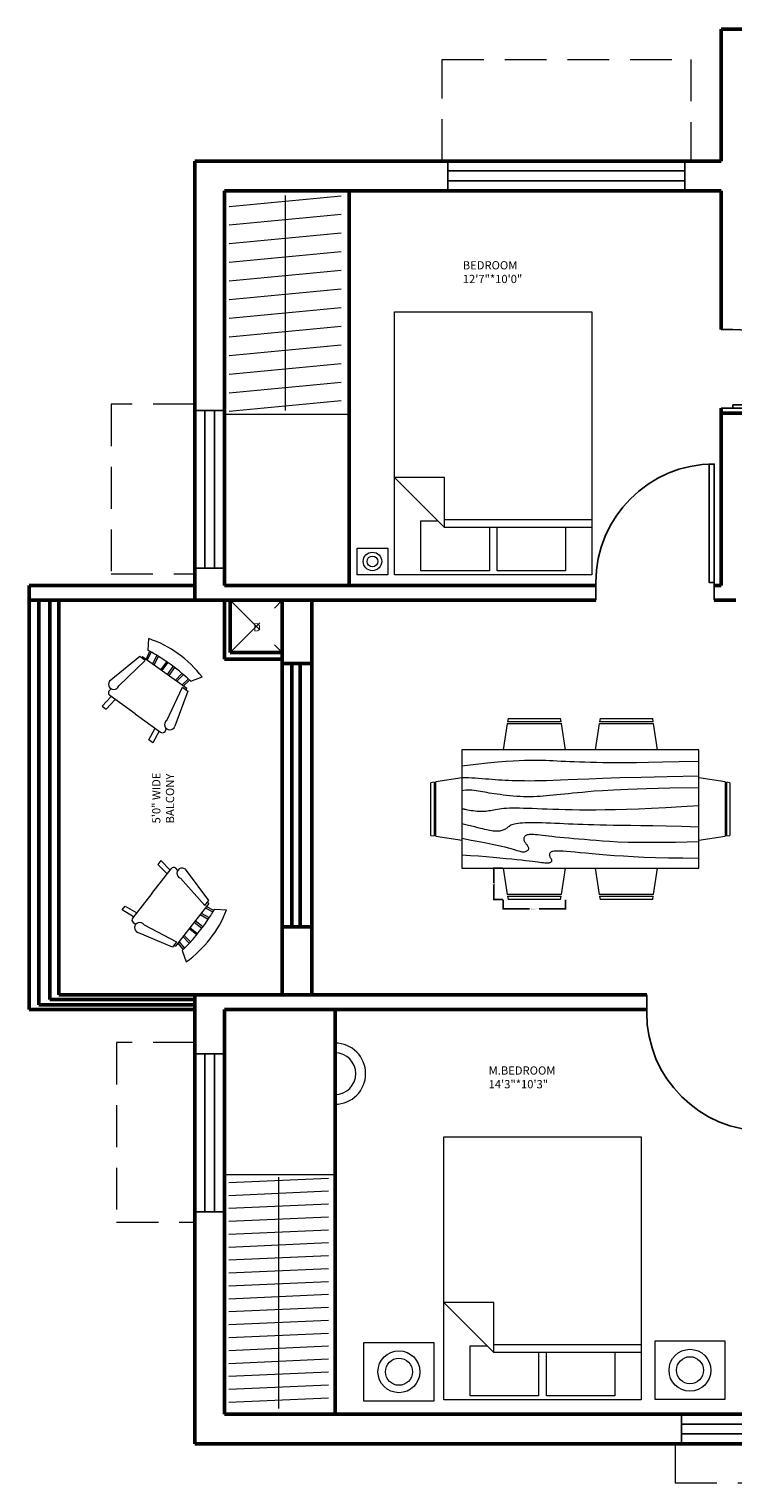
# Model space of a CAD drawing. Units: inches. Extents: x 4795 to 6024, y 2716 to 5025.
# Tile 4 of 19: x 4867 to 5081, y 3339 to 3781. Entities that reach past the tile are written whole.
import ezdxf

# ---------------------------------------------------------------- set-up
doc = ezdxf.new("R2010")
doc.units = ezdxf.units.IN
doc.linetypes.add('DASHED', pattern=[19.05, 12.7, -6.35])
for name, color, linetype, lineweight in [('A-ANNO-DIMS', 2, 'Continuous', 18), ('A-ANNO-TEXT', 7, 'Continuous', 18), ('A-AREA-IDEN', 3, 'Continuous', 18), ('A-DOOR', 4, 'Continuous', 25), ('A-FLOR-FIXT', 9, 'Continuous', 18), ('A-FURN', 8, 'Continuous', 18), ('A-GLAZ', 4, 'Continuous', 25), ('A-WALL', 7, 'Continuous', 50), ('A-WALL-OVHD', 8, 'DASHED', 18)]:
    doc.layers.add(name, color=color, linetype=linetype, lineweight=lineweight)
doc.styles.get("Standard").update_dxf_attribs({"font": 'arial.ttf'})
doc.dimstyles.get("Standard").update_dxf_attribs({"dimtxt": 0.18, "dimasz": 0.18, "dimexe": 0.18, "dimexo": 0.0625, "dimgap": 0.09, "dimtad": 0, "dimtih": 1, "dimtoh": 1, "dimdec": 4, "dimzin": 0, "dimdsep": 46, "dimtxsty": 'Standard', "dimcen": 0.09, "dimadec": 0, "dimazin": 0, "dimtfac": 1, "dimtdec": 4, "dimtofl": 0, "dimtmove": 0, "dimatfit": 3, "dimfxl": 1, "dimtolj": 1, "dimtzin": 0, "dimarcsym": 0})

# ---------------------------------------------------------------- blocks, each defined once
blk = doc.blocks.new('*U2')
for p, q in [((0, 0), (0, -6)), ((40, 0), (40, -6))]:
    blk.add_line(p, q)
blk.add_lwpolyline([(0, 0), (0, 40), (1.75, 40), (1.75, 0)], close=True)
blk.add_arc((0, 0), 40, 0, 90)
blk = doc.blocks.new('Bed - Queen')
for p, q in [((0, -80.00003), (0, 0)), ((0, 0), (59.99999, 0)), ((59.99999, 0), (59.99999, -80.00003)), ((7.99999, -1.2), (28.79998, -1.2)), ((7.99999, -14.4), (7.99999, -1.2)), ((28.79998, -1.2), (28.79998, -14.4)), ((31.19999, -1.2), (51.99999, -1.2)), ((31.19999, -14.4), (31.19999, -1.2)), ((51.99999, -1.2), (51.99999, -16.4)), ((0, -14.4), (44.8, -14.4)), ((44.8, -16.8), (0, -16.8)), ((59.99999, -29.6), (44.8, -14.4)), ((44.8, -14.4), (44.8, -29.6)), ((51.99999, -16.4), (46.79936, -16.4)), ((44.8, -29.6), (59.99999, -29.6)), ((59.99999, -80.00003), (0, -80.00003))]:
    blk.add_line(p, q)
blk = doc.blocks.new('Chair - Rocking')
for p, q in [((-8, -4.5), (-10, -1.5)), ((-4.5, -7), (-4.96674, -4.19951)), ((-4, -7), (-4.40532, -4.16272)), ((-1.5, -4.05012), (-1.5, -7)), ((-1, -7), (-1, -4.05012)), ((1, -7), (1, -4.04655)), ((1.5, -4.05012), (1.5, -7)), ((4, -7), (4.40187, -4.18694)), ((4.5, -7), (4.96761, -4.19437)), ((6.5, -7), (7, -4.4057)), ((8, -4.5), (10, -1.5)), ((-9, -7.5), (-12, -18.49999)), ((-7, -7.5), (-9, -7.5)), ((-9, -18.49999), (-7, -7.5)), ((-8.23428, -6.99939), (-8.3093, -7.47958)), ((-8.23041, -7), (8.23915, -7)), ((-7.5, -4.5), (-7, -7)), ((-6.5, -7), (-7.02225, -4.43)), ((7.5, -4.5), (7, -7)), ((7, -7.5), (9, -7.5)), ((9, -18.49999), (7, -7.5)), ((8.31071, -7.48854), (8.23449, -7.00073)), ((9, -7.5), (12, -18.49999)), ((-10.36644, -20.64523), (-10.5, -21.49999)), ((10.5, -21.49999), (10.3575, -20.58798)), ((-9, -22.49999), (-9.5, -26.49999)), ((0, -22.49999), (-9.5, -22.49999)), ((-9.5, -26.49999), (-8, -26.49999)), ((-8, -26.49999), (-7.5, -22.49999)), ((0, -22.49999), (9.5, -22.49999)), ((8, -26.49999), (7.5, -22.49999)), ((9.5, -26.49999), (8, -26.49999)), ((9, -22.49999), (9.5, -26.49999))]:
    blk.add_line(p, q)
for centre, radius, start, end in [((0, -34.08333), 34.08333, 72.93847, 107.0615), ((0, -68.25004), 64.25, 93.92211, 97.15267), ((0, -68.25004), 64.25, 82.84733, 93.92211), ((-10.5, -18.99999), 1.58114, 161.5651, 18.43495), ((-9.5, -21.49999), 1, 180, 270), ((10.5, -18.99999), 1.58114, 161.5651, 18.43495), ((9.5, -21.49999), 1, 270, 0)]:
    blk.add_arc(centre, radius, start, end)
blk = doc.blocks.new('WIN-48')
for p, q in [((0, 0), (0, 48)), ((0, 48), (9, 48)), ((3, 0), (3, 48)), ((6, 48), (6, 0)), ((9, 48), (9, 0)), ((9, 0), (0, 0))]:
    blk.add_line(p, q)
blk = doc.blocks.new('WIN-72')
for p, q in [((0, 0), (0, 9)), ((0, 9), (72, 9)), ((72, 9), (72, 0)), ((0, 6), (72, 6)), ((72, 3), (0, 3)), ((72, 0), (0, 0))]:
    blk.add_line(p, q)
blk = doc.blocks.new('WIN-24')
for p, q in [((0, 0), (0, 9)), ((0, 9), (24, 9)), ((24, 9), (24, 0)), ((0, 6), (24, 6)), ((24, 3), (0, 3)), ((24, 0), (0, 0))]:
    blk.add_line(p, q)
blk = doc.blocks.new('CHAIR-DINING')
for p, q in [((8, 17.72), (0, 18.97)), ((8, 17.71), (8, 1.25)), ((9.5, 17.48), (8.5, 17.64)), ((8.5, 1.33), (8.5, 17.64)), ((9.5, 17.48), (9.5, 1.48)), ((0, 0), (8, 1.25)), ((8.5, 1.33), (9.5, 1.48))]:
    blk.add_line(p, q)
blk = doc.blocks.new('*D37')
at = {"layer": 'A-ANNO-DIMS', "color": 0, "lineweight": -2, "transparency": 16777216}
for p, q in [((5010.7, 3515.86), (5010.7, 3512.89)), ((5029.67, 3515.86), (5029.67, 3512.89)), ((5010.88, 3513.07), (5018.76, 3513.07)), ((5029.49, 3513.07), (5021.61, 3513.07))]:
    blk.add_line(p, q, dxfattribs=at)
at = {"layer": 'A-ANNO-DIMS', "color": 0, "lineweight": 100, "transparency": 16777216}
for points in [[(5010.88, 3513.1), (5010.88, 3513.04), (5010.7, 3513.07)], [(5029.49, 3513.1), (5029.49, 3513.04), (5029.67, 3513.07)]]:
    blk.add_solid(points, dxfattribs=at)
at = {"layer": 'DEFPOINTS', "color": 0, "lineweight": 100, "transparency": 16777216}
for p in [(5010.7, 3515.92), (5029.67, 3515.92), (5029.67, 3513.07)]:
    blk.add_point(p, dxfattribs=at)
at = {"layer": 'A-ANNO-DIMS', "color": 0, "transparency": 16777216, "insert": (5020.18, 3513.07), "char_height": 0.18, "attachment_point": 5}
blk.add_mtext('\\A1;DINING CHAIR 19 TYP.', dxfattribs=at)
blk = doc.blocks.new('*D38')
at = {"layer": 'A-ANNO-DIMS', "color": 0, "lineweight": -2, "transparency": 16777216}
for p, q in [((5010.64, 3525.42), (5007.67, 3525.42)), ((5007.85, 3525.24), (5007.85, 3520.85)), ((5007.85, 3516.1), (5007.85, 3520.49)), ((5010.64, 3515.92), (5007.67, 3515.92))]:
    blk.add_line(p, q, dxfattribs=at)
at = {"layer": 'A-ANNO-DIMS', "color": 0, "lineweight": 100, "transparency": 16777216}
for points in [[(5007.82, 3525.24), (5007.88, 3525.24), (5007.85, 3525.42)], [(5007.82, 3516.1), (5007.88, 3516.1), (5007.85, 3515.92)]]:
    blk.add_solid(points, dxfattribs=at)
at = {"layer": 'DEFPOINTS', "color": 0, "lineweight": 100, "transparency": 16777216}
for p in [(5010.7, 3525.42), (5007.85, 3515.92), (5010.7, 3515.92)]:
    blk.add_point(p, dxfattribs=at)
at = {"layer": 'A-ANNO-DIMS', "color": 0, "transparency": 16777216, "insert": (5007.85, 3520.67), "char_height": 0.18, "attachment_point": 5}
blk.add_mtext('\\A1;10 TYP.', dxfattribs=at)

msp = doc.modelspace()

# ---------------------------------------------------------------- linework, layer by layer
at = {"layer": 'A-FLOR-FIXT'}
msp.add_lwpolyline([(4975.61, 3614.64), (4966.31, 3614.64), (4966.31, 3622.77), (4975.61, 3622.77)], close=True, dxfattribs=at)
for radius in [2.81, 1.65]:
    msp.add_circle((4970.96, 3618.7), radius, dxfattribs=at)
at = {"layer": 'A-FURN'}
for p, q in [((4927.43, 3726.67), (4961.4, 3729.91)), ((4944.42, 3730.01), (4944.42, 3664.56)), ((4927.43, 3721), (4961.4, 3724.24)), ((4927.43, 3715.34), (4961.4, 3718.58)), ((4927.43, 3709.67), (4961.4, 3712.91)), ((4927.43, 3704.01), (4961.4, 3707.25)), ((4927.43, 3698.34), (4961.4, 3701.58)), ((4927.43, 3692.67), (4961.4, 3695.92)), ((4927.43, 3687.01), (4961.4, 3690.25)), ((4927.43, 3681.34), (4961.4, 3684.59)), ((4927.43, 3675.68), (4961.4, 3678.92)), ((4927.43, 3670.01), (4961.4, 3673.25)), ((4927.43, 3664.35), (4961.4, 3667.59)), ((4925.97, 3663.46), (4963.83, 3663.46)), ((5070.18, 3561.42), (4998.18, 3561.42)), ((4998.18, 3561.42), (4998.18, 3525.42)), ((5070.18, 3525.42), (5070.18, 3561.42)), ((4989.69, 3551.58), (4988.68, 3551.42)), ((4988.68, 3535.42), (4988.68, 3551.42)), ((4989.68, 3551.58), (4989.68, 3535.27)), ((4990.18, 3535.19), (4990.18, 3551.66)), ((4998.19, 3552.9), (4990.19, 3551.65)), ((4988.68, 3535.42), (4989.68, 3535.26)), ((4990.18, 3535.19), (4998.19, 3533.93)), ((4998.18, 3525.42), (5070.18, 3525.42)), ((4925.97, 3432.32), (4959.59, 3432.32)), ((4927.31, 3429.9), (4957.55, 3431.24)), ((4942.43, 3431.54), (4942.43, 3361.15)), ((4927.31, 3425.97), (4957.55, 3427.31)), ((4927.31, 3422.04), (4957.55, 3423.38)), ((4927.31, 3418.11), (4957.55, 3419.45)), ((4927.31, 3414.18), (4957.55, 3415.53)), ((4927.31, 3410.25), (4957.55, 3411.6)), ((4927.31, 3406.32), (4957.55, 3407.67)), ((4927.31, 3402.4), (4957.55, 3403.74)), ((4927.31, 3398.47), (4957.55, 3399.81)), ((4927.31, 3394.54), (4957.55, 3395.88)), ((4927.31, 3390.61), (4957.55, 3391.95)), ((4927.31, 3386.68), (4957.55, 3388.02)), ((4927.31, 3382.75), (4957.55, 3384.1)), ((4927.31, 3378.82), (4957.55, 3380.17)), ((4927.31, 3374.89), (4957.55, 3376.24)), ((4927.31, 3370.97), (4957.55, 3372.31)), ((4927.31, 3367.04), (4957.55, 3368.38)), ((4927.31, 3363.11), (4957.55, 3364.45))]:
    msp.add_line(p, q, dxfattribs=at)
for points in [[(5070.18, 3557.92), (5064.27, 3557.75), (5059.22, 3557.63), (5054.92, 3557.55), (5051.26, 3557.49), (5048.15, 3557.47), (5045.49, 3557.46), (5043.16, 3557.48), (5041.06, 3557.5), (5039.11, 3557.54), (5037.28, 3557.58), (5035.56, 3557.63), (5033.94, 3557.68), (5032.42, 3557.74), (5030.99, 3557.8), (5029.63, 3557.86), (5028.35, 3557.92), (5027.13, 3557.98), (5025.95, 3558.04), (5024.79, 3558.1), (5023.64, 3558.14), (5022.47, 3558.18), (5021.26, 3558.21), (5019.99, 3558.22), (5018.64, 3558.21), (5017.19, 3558.18), (5015.57, 3558.12), (5013.7, 3558.02), (5011.52, 3557.86), (5008.95, 3557.63), (5005.92, 3557.33), (5002.36, 3556.93), (4998.18, 3556.42)], [(5070.18, 3553.42), (5060.59, 3553.23), (5052.65, 3553.05), (5046.17, 3552.87), (5040.92, 3552.7), (5036.71, 3552.54), (5033.31, 3552.4), (5030.51, 3552.27), (5028.1, 3552.17), (5025.91, 3552.09), (5023.88, 3552.03), (5022.01, 3551.99), (5020.29, 3551.96), (5018.7, 3551.95), (5017.23, 3551.96), (5015.87, 3551.98), (5014.6, 3552), (5013.42, 3552.04), (5012.32, 3552.08), (5011.27, 3552.13), (5010.26, 3552.19), (5009.28, 3552.25), (5008.31, 3552.31), (5007.34, 3552.39), (5006.35, 3552.46), (5005.34, 3552.54), (5004.3, 3552.62), (5003.25, 3552.7), (5002.21, 3552.77), (5001.16, 3552.83), (5000.14, 3552.88), (4999.14, 3552.91), (4998.18, 3552.92)], [(5070.18, 3549.92), (5061.37, 3549.73), (5054.27, 3549.55), (5048.65, 3549.36), (5044.29, 3549.18), (5040.96, 3549), (5038.42, 3548.83), (5036.45, 3548.66), (5034.81, 3548.5), (5033.31, 3548.35), (5031.91, 3548.21), (5030.6, 3548.07), (5029.36, 3547.94), (5028.18, 3547.82), (5027.06, 3547.71), (5025.98, 3547.6), (5024.93, 3547.5), (5023.91, 3547.41), (5022.91, 3547.33), (5021.92, 3547.27), (5020.93, 3547.21), (5019.95, 3547.17), (5018.96, 3547.15), (5017.96, 3547.15), (5016.93, 3547.17), (5015.89, 3547.21), (5014.84, 3547.28), (5013.78, 3547.36), (5012.74, 3547.45), (5011.71, 3547.56), (5010.71, 3547.67), (5009.76, 3547.8), (5008.85, 3547.92), (5008.01, 3548.04), (5007.22, 3548.17), (5006.47, 3548.29), (5005.76, 3548.41), (5005.08, 3548.53), (5004.43, 3548.65), (5003.78, 3548.77), (5003.14, 3548.88), (5002.5, 3548.98), (5001.86, 3549.08), (5001.22, 3549.15), (5000.59, 3549.2), (4999.96, 3549.2), (4999.35, 3549.17), (4998.76, 3549.07), (4998.18, 3548.92)], [(5070.18, 3544.42), (5064.98, 3544.08), (5060.2, 3543.8), (5055.84, 3543.58), (5051.84, 3543.41), (5048.19, 3543.29), (5044.84, 3543.21), (5041.76, 3543.15), (5038.93, 3543.13), (5036.32, 3543.12), (5033.9, 3543.13), (5031.65, 3543.16), (5029.57, 3543.2), (5027.63, 3543.24), (5025.82, 3543.3), (5024.12, 3543.36), (5022.52, 3543.42), (5021, 3543.48), (5019.55, 3543.54), (5018.19, 3543.59), (5016.9, 3543.64), (5015.7, 3543.67), (5014.58, 3543.69), (5013.55, 3543.69), (5012.6, 3543.67), (5011.74, 3543.63), (5010.95, 3543.57), (5010.23, 3543.49), (5009.57, 3543.4), (5008.96, 3543.3), (5008.39, 3543.2), (5007.86, 3543.1), (5007.35, 3543), (5006.86, 3542.91), (5006.38, 3542.83), (5005.9, 3542.77), (5005.41, 3542.71), (5004.92, 3542.67), (5004.42, 3542.65), (5003.9, 3542.65), (5003.35, 3542.67), (5002.78, 3542.71), (5002.19, 3542.77), (5001.6, 3542.85), (5001.02, 3542.93), (5000.48, 3543.02), (4999.99, 3543.1), (4999.57, 3543.18), (4999.23, 3543.25), (4998.98, 3543.31), (4998.8, 3543.35), (4998.68, 3543.38), (4998.6, 3543.4), (4998.53, 3543.41), (4998.45, 3543.42), (4998.34, 3543.42), (4998.18, 3543.42)], [(5070.18, 3537.92), (5064.9, 3538.08), (5060.25, 3538.21), (5056.18, 3538.3), (5052.61, 3538.37), (5049.49, 3538.41), (5046.74, 3538.45), (5044.3, 3538.47), (5042.1, 3538.5), (5040.09, 3538.54), (5038.24, 3538.58), (5036.53, 3538.63), (5034.92, 3538.68), (5033.41, 3538.74), (5031.96, 3538.8), (5030.56, 3538.86), (5029.18, 3538.92), (5027.81, 3538.98), (5026.45, 3539.04), (5025.11, 3539.1), (5023.81, 3539.15), (5022.55, 3539.19), (5021.36, 3539.22), (5020.23, 3539.25), (5019.18, 3539.25), (5018.23, 3539.25), (5017.37, 3539.22), (5016.58, 3539.18), (5015.88, 3539.13), (5015.26, 3539.06), (5014.7, 3538.97), (5014.2, 3538.87), (5013.77, 3538.75), (5013.39, 3538.62), (5013.05, 3538.48), (5012.76, 3538.32), (5012.5, 3538.16), (5012.26, 3537.99), (5012.03, 3537.83), (5011.82, 3537.66), (5011.6, 3537.5), (5011.38, 3537.35), (5011.14, 3537.21), (5010.9, 3537.08), (5010.63, 3536.96), (5010.35, 3536.86), (5010.04, 3536.78), (5009.71, 3536.71), (5009.35, 3536.67), (5008.96, 3536.65), (5008.54, 3536.65), (5008.1, 3536.68), (5007.63, 3536.72), (5007.15, 3536.79), (5006.64, 3536.87), (5006.13, 3536.97), (5005.6, 3537.09), (5005.06, 3537.22), (5004.48, 3537.37), (5003.82, 3537.55), (5003.05, 3537.75), (5002.14, 3537.99), (5001.04, 3538.26), (4999.74, 3538.57), (4998.18, 3538.92)], [(5070.18, 3533.42), (5063.16, 3533.28), (5057.36, 3533.22), (5052.61, 3533.22), (5048.75, 3533.28), (5045.62, 3533.39), (5043.06, 3533.53), (5040.9, 3533.68), (5038.98, 3533.84), (5037.15, 3533.99), (5035.41, 3534.13), (5033.74, 3534.27), (5032.16, 3534.41), (5030.66, 3534.54), (5029.24, 3534.67), (5027.92, 3534.79), (5026.68, 3534.92), (5025.54, 3535.04), (5024.49, 3535.17), (5023.53, 3535.28), (5022.65, 3535.39), (5021.86, 3535.48), (5021.14, 3535.56), (5020.5, 3535.63), (5019.93, 3535.67), (5019.44, 3535.69), (5019.01, 3535.69), (5018.63, 3535.66), (5018.31, 3535.62), (5018.04, 3535.55), (5017.8, 3535.47), (5017.6, 3535.37), (5017.43, 3535.25), (5017.29, 3535.12), (5017.17, 3534.97), (5017.08, 3534.82), (5017.01, 3534.65), (5016.97, 3534.47), (5016.95, 3534.29), (5016.97, 3534.11), (5017.02, 3533.92), (5017.1, 3533.73), (5017.2, 3533.54), (5017.32, 3533.36), (5017.46, 3533.17), (5017.6, 3532.98), (5017.74, 3532.79), (5017.89, 3532.61), (5018.02, 3532.42), (5018.13, 3532.23), (5018.23, 3532.05), (5018.31, 3531.86), (5018.36, 3531.68), (5018.39, 3531.5), (5018.38, 3531.33), (5018.34, 3531.16), (5018.27, 3531), (5018.16, 3530.85), (5018.01, 3530.71), (5017.82, 3530.59), (5017.61, 3530.48), (5017.37, 3530.4), (5017.11, 3530.35), (5016.82, 3530.32), (5016.52, 3530.34), (5016.2, 3530.39), (5015.84, 3530.47), (5015.45, 3530.59), (5014.99, 3530.74), (5014.47, 3530.91), (5013.85, 3531.1), (5013.14, 3531.32), (5012.31, 3531.54), (5011.35, 3531.79), (5010.23, 3532.05), (5008.91, 3532.33), (5007.36, 3532.65), (5005.54, 3533.02), (5003.43, 3533.43), (5000.99, 3533.89), (4998.18, 3534.42)], [(5070.18, 3528.42), (5065.36, 3528.44), (5060.99, 3528.51), (5057.04, 3528.6), (5053.46, 3528.73), (5050.22, 3528.88), (5047.28, 3529.05), (5044.6, 3529.23), (5042.14, 3529.42), (5039.88, 3529.61), (5037.79, 3529.79), (5035.88, 3529.96), (5034.15, 3530.13), (5032.59, 3530.28), (5031.2, 3530.4), (5029.99, 3530.51), (5028.93, 3530.59), (5028.05, 3530.63), (5027.3, 3530.65), (5026.7, 3530.64), (5026.21, 3530.61), (5025.82, 3530.55), (5025.51, 3530.47), (5025.28, 3530.37), (5025.1, 3530.25), (5024.96, 3530.12), (5024.86, 3529.98), (5024.8, 3529.82), (5024.76, 3529.66), (5024.75, 3529.49), (5024.76, 3529.33), (5024.8, 3529.16), (5024.85, 3529), (5024.92, 3528.85), (5025, 3528.7), (5025.09, 3528.56), (5025.17, 3528.43), (5025.26, 3528.3), (5025.33, 3528.17), (5025.39, 3528.04), (5025.43, 3527.92), (5025.45, 3527.79), (5025.45, 3527.67), (5025.42, 3527.55), (5025.37, 3527.44), (5025.3, 3527.34), (5025.2, 3527.24), (5025.08, 3527.16), (5024.93, 3527.09), (5024.77, 3527.03), (5024.57, 3526.99), (5024.33, 3526.97), (5024.06, 3526.96), (5023.74, 3526.97), (5023.36, 3526.99), (5022.93, 3527.03), (5022.43, 3527.09), (5021.87, 3527.16), (5021.22, 3527.24), (5020.47, 3527.34), (5019.62, 3527.45), (5018.65, 3527.57), (5017.54, 3527.71), (5016.3, 3527.85), (5014.89, 3528), (5013.33, 3528.16), (5011.6, 3528.33), (5009.71, 3528.5), (5007.68, 3528.68), (5005.5, 3528.86), (5003.19, 3529.05), (5000.75, 3529.23), (4998.18, 3529.42)]]:
    msp.add_lwpolyline(points, dxfattribs=at)
for points in [[(5056.88, 3381.72), (5078.14, 3381.72), (5078.14, 3363.89), (5056.88, 3363.89)], [(4968.37, 3381.24), (4989.63, 3381.24), (4989.63, 3363.41), (4968.37, 3363.41)]]:
    msp.add_lwpolyline(points, close=True, dxfattribs=at)
for centre, radius in [((4979, 3372.33), 6.37), ((5067.51, 3372.8), 6.37), ((4979, 3372.33), 4.11), ((5067.51, 3372.8), 4.11)]:
    msp.add_circle(centre, radius, dxfattribs=at)
for radius in [9.3, 6.32]:
    msp.add_arc((4959.59, 3462.97), radius, 270, 90, dxfattribs=at)
at = {"layer": 'A-WALL'}
for p, q in [((5076.97, 3740.43), (5076.97, 3780.56)), ((5076.97, 3780.56), (5151.39, 3780.56)), ((4916.97, 3740.43), (4916.97, 3606.93)), ((5076.97, 3740.43), (4916.97, 3740.43)), ((4925.97, 3731.43), (4925.97, 3611.43)), ((5076.97, 3731.43), (4925.97, 3731.43)), ((4963.83, 3731.43), (4963.83, 3611.43)), ((5076.97, 3731.43), (5076.97, 3689.26)), ((5076.97, 3665.26), (5076.97, 3611.43)), ((5076.97, 3663.74), (5141.47, 3663.74)), ((4916.97, 3611.43), (4866.53, 3611.43)), ((4866.53, 3611.43), (4866.53, 3606.93)), ((5038.88, 3611.43), (4925.97, 3611.43)), ((5076.97, 3611.43), (5074.88, 3611.43)), ((4866.53, 3606.93), (4866.53, 3486.93)), ((4875.53, 3606.93), (4866.53, 3606.93)), ((4869.47, 3606.93), (4869.47, 3483.87)), ((4872.88, 3606.93), (4872.88, 3485.48)), ((4875.53, 3606.93), (4875.53, 3486.93)), ((4916.97, 3606.93), (4875.53, 3606.93)), ((5038.88, 3606.93), (4916.97, 3606.93)), ((4925.97, 3606.93), (4925.97, 3588.99)), ((4927.72, 3606.93), (4927.72, 3590.98)), ((4943.53, 3606.93), (4943.53, 3486.93)), ((4952.53, 3606.93), (4952.53, 3486.93)), ((5081.47, 3606.93), (5074.88, 3606.93)), ((4927.72, 3590.98), (4943.53, 3590.98)), ((4925.97, 3588.99), (4943.53, 3588.99)), ((4943.53, 3587.66), (4952.53, 3587.66)), ((4946.44, 3587.66), (4946.44, 3507.57)), ((4949.01, 3587.66), (4949.01, 3507.57)), ((4943.53, 3507.57), (4952.53, 3507.57)), ((4866.53, 3482.43), (4866.53, 3486.93)), ((4869.47, 3483.87), (4916.97, 3483.87)), ((4872.88, 3485.48), (4916.97, 3485.48)), ((4916.97, 3486.93), (4875.53, 3486.93)), ((4916.97, 3486.93), (4916.97, 3350.43)), ((5054.35, 3486.93), (4916.97, 3486.93)), ((4916.97, 3482.43), (4866.53, 3482.43)), ((4925.97, 3482.43), (4925.97, 3359.43)), ((5054.35, 3482.43), (4925.97, 3482.43)), ((4959.59, 3482.43), (4959.59, 3359.43)), ((5096.97, 3359.43), (4925.97, 3359.43)), ((5096.97, 3350.43), (4916.97, 3350.43))]:
    msp.add_line(p, q, dxfattribs=at)
at = {"layer": 'A-WALL-OVHD'}
for p, q in [((4992.13, 3740.43), (4992.13, 3771.34)), ((4992.13, 3771.34), (5067.74, 3771.34)), ((5067.74, 3771.34), (5067.74, 3740.43)), ((4916.97, 3666.5), (4891.51, 3666.5)), ((4891.51, 3666.5), (4891.51, 3614.91)), ((4891.51, 3614.91), (4916.97, 3614.91)), ((4927.72, 3606.93), (4943.53, 3590.98)), ((4927.72, 3590.98), (4943.53, 3606.93)), ((4916.97, 3472.42), (4893.14, 3472.42)), ((4893.14, 3472.42), (4893.14, 3417.78)), ((4893.14, 3417.78), (4916.97, 3417.78)), ((5062.99, 3350.43), (5062.99, 3338.54)), ((5062.99, 3338.54), (5090.95, 3338.54))]:
    msp.add_line(p, q, dxfattribs=at)

# ---------------------------------------------------------------- block references
at = {"layer": 'A-DOOR'}
for p, xscale, yscale, zscale, rotation in [((5080.57, 3665.26), -0.6, 0.6, 0.6, 270), ((5090.35, 3481.53), 0.9, 0.9, 0.9, 180)]:
    msp.add_blockref('*U2', p, dxfattribs=dict(at, xscale=xscale, yscale=yscale, zscale=zscale, rotation=rotation))
at = {"layer": 'A-DOOR', "xscale": -0.9, "yscale": 0.9, "zscale": 0.9}
msp.add_blockref('*U2', (5074.88, 3612.33), dxfattribs=at)
at = {"layer": 'A-FURN'}
for name, p, rotation in [('Bed - Queen', (5037.71, 3614.64), 180), ('Chair - Rocking', (4911.9, 3590.63), 324.2775344515209), ('CHAIR-DINING', (5029.67, 3561.42), 90.0056718244202), ('CHAIR-DINING', (5057.67, 3561.42), 90.0056718244202), ('CHAIR-DINING', (5070.18, 3533.94), 0.0058497063858154), ('Chair - Rocking', (4921.6, 3503.93), 232.0049313276433), ('CHAIR-DINING', (5010.7, 3525.42), 270.0000000000017), ('CHAIR-DINING', (5038.7, 3525.42), 270.0000000000027), ('Bed - Queen', (5052.67, 3363.78), 180)]:
    msp.add_blockref(name, p, dxfattribs=dict(at, rotation=rotation))
at = {"layer": 'A-GLAZ', "rotation": 180}
for name, p in [('WIN-72', (5065.92, 3740.43)), ('WIN-48', (4925.97, 3664.64)), ('WIN-48', (4925.97, 3469.01)), ('WIN-24', (5088.95, 3359.43))]:
    msp.add_blockref(name, p, dxfattribs=at)

# ---------------------------------------------------------------- texts
at = {"layer": 'A-ANNO-TEXT', "insert": (4934.65, 3599.93), "char_height": 2.5, "attachment_point": 1}
msp.add_mtext_dynamic_manual_height_columns('D', width=2.2755, gutter_width=12.5, heights=[0], dxfattribs=at)
at = {"layer": 'A-AREA-IDEN', "char_height": 2.5, "attachment_point": 1}
for s, width, insert in [('BEDROOM\\P12\'7"*10\'0"', 54.9037, (4998.43, 3710)), ('M.BEDROOM\\P14\'3"*10\'3"', 57.0139, (5006.29, 3465.18))]:
    msp.add_mtext_dynamic_manual_height_columns(s, width=width, gutter_width=12.5, heights=[0], dxfattribs=dict(at, insert=insert))
at = {"layer": 'A-AREA-IDEN', "insert": (4903.97, 3539.05), "char_height": 2.5, "attachment_point": 1, "rotation": 90}
msp.add_mtext_dynamic_manual_height_columns('5\'0" WIDE\\PBALCONY', width=41.122, gutter_width=12.5, heights=[0], dxfattribs=at)

# ---------------------------------------------------------------- dimensions: what is measured, and where the dimension line sits
at = {"layer": 'A-ANNO-DIMS'}
for base, p1, p2, angle, text, picture, middle in [((5007.8547, 3515.9196), (5010.7001, 3525.422), (5010.7001, 3515.9196), 270, '<> TYP.', '*D38', (5007.8547, 3520.6708)), ((5029.67, 3513.07), (5010.7, 3515.92), (5029.67, 3515.92), 0, 'DINING CHAIR <> TYP.', '*D37', (5020.18, 3513.07))]:
    dim = msp.add_linear_dim(base=base, p1=p1, p2=p2, angle=angle, text=text, dimstyle='Standard', override={"dimdec": 0, "dimlfac": 1, "dimrnd": 0, "dimzin": 0, "dimdsep": 46, "dimlunit": 2}, dxfattribs=at)
    dim.commit()
    dim.dimension.update_dxf_attribs({"geometry": picture, "text_midpoint": middle})

doc.saveas('drawing.dxf')
